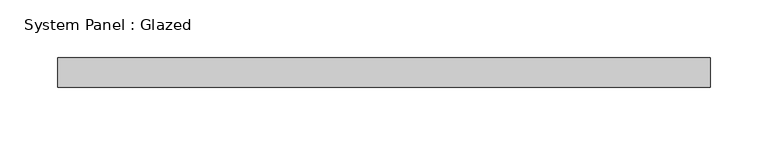
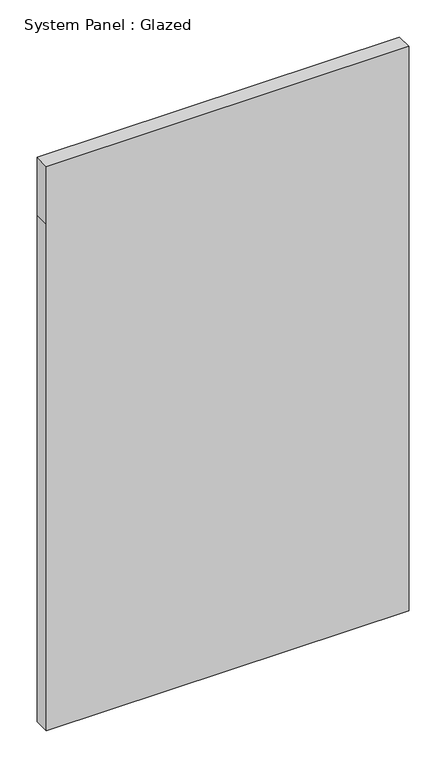
"""IFC4 building model written with IfcOpenShell, lengths in millimetres: plate geometry, System Panel : Glazed."""

from ifc_helpers import new_model, si_unit, frame, origin, place, context, project, spatial, polyline, outline, extrude, source, transform, mapped, element, save


def system_panel_glazed_48a86efd(model_context):
    return source(origin(), model_context, "Body", "SweptSolid", [
        extrude(outline(polyline([(0.0, -282.575), (0.0, 282.575), (833.9039078, 282.575), (929.1539078, 282.575), (929.1539078, -282.575), (833.9039078, -282.575), (0.0, -282.575)])), frame((0.0, 19.05, 0.0), z_axis=(0.0, 1.0, 0.0), x_axis=(0.0, 0.0, 1.0)), (0.0, 0.0, 1.0), 25.4),
    ])


if __name__ == "__main__":
    model = new_model("IFC4")
    model_context = context("Model", 3, world=origin())
    ifc_project = project(units=[si_unit("LENGTHUNIT", "METRE", prefix="MILLI")], contexts=[model_context])
    site = spatial("IfcSite", under=ifc_project)
    building = spatial("IfcBuilding", under=site)
    placement = place(None, origin())
    system_panel_glazed_shape = system_panel_glazed_48a86efd(model_context)
    element("IfcPlate", 1, ObjectType="System Panel : Glazed", at=placement, inside=building, context=model_context, shape_type="MappedRepresentation", body=[
        mapped(system_panel_glazed_shape, transform((0.0, 0.0, 0.0), x_axis=(1.0, 0.0, 0.0), y_axis=(0.0, 1.0, 0.0), z_axis=(0.0, 0.0, 1.0))),
    ])
    save(model, "model.ifc")

# Revit data of these elements
# Type "System Panel : Glazed"
#   Construction Type Id = "GSP4R"
#   Analytic Construction = "1/8 in Pilkington single glazing"
#   Visual Light Transmittance = 0.9
#   Solar Heat Gain Coefficient = 0.86
#   Heat Transfer Coefficient (U) = 1.18115 BTU/(h·ft²·°F)
#   Define Thermal Properties by = 1
# Element 1 (IfcPlate, "System Panel : Glazed")
#   Materials on its faces: "Glass"
# Materials
#   "Glass": class "Glass", colour RGB 0 128 192, transparency 0.75, Description = "Soda Lime Glass", Cost = 0
